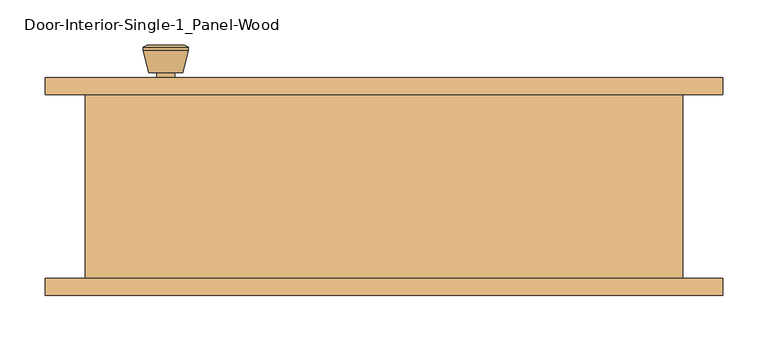
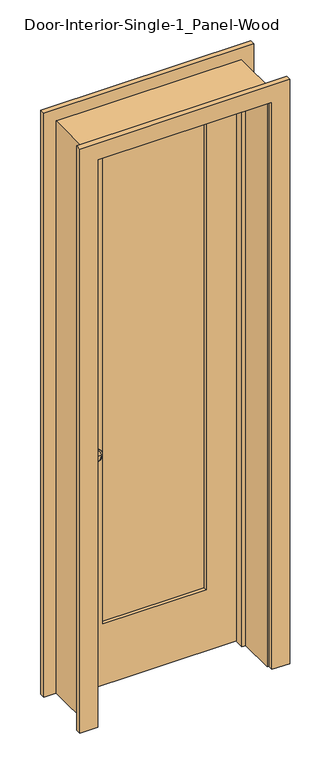
"""IFC4 building model written with IfcOpenShell, lengths in millimetres: door geometry, Door-Interior-Single-1_Panel-Wood."""

from ifc_helpers import new_model, si_unit, point, frame, frame_2d, origin, place, context, project, spatial, polyline, circle_curve, trimmed, segment, composite_curve, outline, extrude, faceted_brep, source, transform, mapped, element, save
from ifc_brep_helpers import plane_surface, cylinder_surface, revolved_surface, advanced_brep


def door_interior_single_1_panel_wood_5fe0af8f(model_context):
    return source(origin(), model_context, "Body", "SolidModel", [
        advanced_brep(
        [(-241.3, 57.5, 914.4), (-231.3, 57.5, 914.4), (-251.3, 57.5, 914.4), (-220.8241324, 8.5, 914.4), (-241.3, 8.5, 914.4), (-261.7758676, 8.5, 914.4), (-216.3, 10.3278681, 914.4), (-266.3, 10.3278681, 914.4), (-216.3, 13.7915463, 914.4), (-266.3, 13.7915463, 914.4), (-222.663764, 38.5, 914.4), (-259.936236, 38.5, 914.4), (-231.3, 38.5, 914.4), (-251.3, 38.5, 914.4)],
        [
            (0, 1),
            (1, 2, circle_curve(frame((-241.3, 57.5, 914.4), z_axis=(0.0, 1.0, 0.0), x_axis=(-1.0, 0.0, 0.0)), 10.0)),
            (2, 0),
            (2, 1, circle_curve(frame((-241.3, 57.5, 914.4), z_axis=(0.0, 1.0, 0.0), x_axis=(-1.0, 0.0, 0.0)), 10.0)),
            (3, 4),
            (4, 5),
            (5, 3, circle_curve(frame((-241.3, 8.5, 914.4), z_axis=(0.0, -1.0, 0.0), x_axis=(-1.0, 0.0, 0.0)), 20.4758676)),
            (3, 5, circle_curve(frame((-241.3, 8.5, 914.4), z_axis=(0.0, -1.0, 0.0), x_axis=(-1.0, 0.0, 0.0)), 20.4758676)),
            (6, 3),
            (5, 7),
            (7, 6, circle_curve(frame((-241.3, 10.3278681, 914.4), z_axis=(0.0, -1.0, 0.0), x_axis=(-1.0, 0.0, 0.0)), 25.0)),
            (6, 7, circle_curve(frame((-241.3, 10.3278681, 914.4), z_axis=(0.0, -1.0, 0.0), x_axis=(-1.0, 0.0, 0.0)), 25.0)),
            (8, 6),
            (7, 9),
            (9, 8, circle_curve(frame((-241.3, 13.7915463, 914.4), z_axis=(0.0, -1.0, 0.0), x_axis=(-1.0, 0.0, 0.0)), 25.0)),
            (8, 9, circle_curve(frame((-241.3, 13.7915463, 914.4), z_axis=(0.0, -1.0, 0.0), x_axis=(-1.0, 0.0, 0.0)), 25.0)),
            (10, 8),
            (9, 11),
            (11, 10, circle_curve(frame((-241.3, 38.5, 914.4), z_axis=(0.0, -1.0, 0.0), x_axis=(-1.0, 0.0, 0.0)), 18.636236)),
            (10, 11, circle_curve(frame((-241.3, 38.5, 914.4), z_axis=(0.0, -1.0, 0.0), x_axis=(-1.0, 0.0, 0.0)), 18.636236)),
            (12, 10),
            (11, 13),
            (13, 12, circle_curve(frame((-241.3, 38.5, 914.4), z_axis=(0.0, -1.0, 0.0), x_axis=(-1.0, 0.0, 0.0)), 10.0)),
            (12, 13, circle_curve(frame((-241.3, 38.5, 914.4), z_axis=(0.0, -1.0, 0.0), x_axis=(-1.0, 0.0, 0.0)), 10.0)),
            (1, 12),
            (13, 2),
        ],
        [
            plane_surface(frame((-241.3, 57.5, 914.4), z_axis=(0.0, 1.0, 0.0), x_axis=(-1.0, 0.0, 0.0))),
            plane_surface(frame((-241.3, 8.5, 914.4), z_axis=(0.0, -1.0, 0.0), x_axis=(-1.0, 0.0, 0.0))),
            revolved_surface(polyline([(-261.7758676, 8.5, 914.4), (-266.3, 10.3278681, 914.4)]), (-241.3, 57.5, 914.4), (0.0, 1.0, 0.0)),
            cylinder_surface(frame((-241.3, 57.5, 914.4), z_axis=(0.0, 1.0, 0.0), x_axis=(-1.0, 0.0, 0.0)), 25.0),
            revolved_surface(polyline([(-266.3, 13.7915463, 914.4), (-259.936236, 38.5, 914.4)]), (-241.3, 57.5, 914.4), (0.0, 1.0, 0.0)),
            plane_surface(frame((-241.3, 38.5, 914.4), z_axis=(0.0, 1.0, 0.0), x_axis=(-1.0, 0.0, 0.0))),
            cylinder_surface(frame((-241.3, 57.5, 914.4), z_axis=(0.0, 1.0, 0.0), x_axis=(-1.0, 0.0, 0.0)), 10.0),
        ],
        [
            (0, [[1, 2, 3]]),
            (0, [[-3, 4, -1]]),
            (1, [[5, 6, 7]]),
            (1, [[-6, -5, 8]]),
            (2, [[9, -7, 10, 11]]),
            (2, [[-10, -8, -9, 12]]),
            (3, [[13, -11, 14, 15]]),
            (3, [[-14, -12, -13, 16]]),
            (4, [[17, -15, 18, 19]]),
            (4, [[-18, -16, -17, 20]]),
            (5, [[21, -19, 22, 23]]),
            (5, [[-22, -20, -21, 24]]),
            (6, [[25, -23, 26, -2]]),
            (6, [[-26, -24, -25, -4]]),
        ],
    ),
        extrude(outline(composite_curve([segment(trimmed(circle_curve(frame_2d((914.4, -241.3)), 30.0), [point((914.4, -271.3))], [point((914.4, -211.3))], False, "CARTESIAN"), True, "CONTINUOUS"), segment(trimmed(circle_curve(frame_2d((914.4, -241.3)), 30.0), [point((914.4, -211.3))], [point((914.4, -271.3))], False, "CARTESIAN"), True, "CONTINUOUS")], self_intersect=False)), frame((0.0, 57.5, 0.0), z_axis=(0.0, 1.0, 0.0), x_axis=(0.0, 0.0, 1.0)), (0.0, 0.0, 1.0), 6.0),
        advanced_brep(
        [(-241.3, 104.425, 914.4), (-251.3, 104.425, 914.4), (-231.3, 104.425, 914.4), (-220.8241324, 153.425, 914.4), (-261.7758676, 153.425, 914.4), (-241.3, 153.425, 914.4), (-216.3, 151.5971319, 914.4), (-266.3, 151.5971319, 914.4), (-216.3, 148.1334537, 914.4), (-266.3, 148.1334537, 914.4), (-222.663764, 123.425, 914.4), (-259.936236, 123.425, 914.4), (-231.3, 123.425, 914.4), (-251.3, 123.425, 914.4)],
        [
            (0, 1),
            (1, 2, circle_curve(frame((-241.3, 104.425, 914.4), z_axis=(0.0, -1.0, 0.0), x_axis=(-1.0, 0.0, 0.0)), 10.0)),
            (2, 0),
            (2, 1, circle_curve(frame((-241.3, 104.425, 914.4), z_axis=(0.0, -1.0, 0.0), x_axis=(-1.0, 0.0, 0.0)), 10.0)),
            (3, 4, circle_curve(frame((-241.3, 153.425, 914.4), z_axis=(0.0, 1.0, 0.0), x_axis=(-1.0, 0.0, 0.0)), 20.4758676)),
            (4, 5),
            (5, 3),
            (4, 3, circle_curve(frame((-241.3, 153.425, 914.4), z_axis=(0.0, 1.0, 0.0), x_axis=(-1.0, 0.0, 0.0)), 20.4758676)),
            (6, 7, circle_curve(frame((-241.3, 151.5971319, 914.4), z_axis=(0.0, 1.0, 0.0), x_axis=(-1.0, 0.0, 0.0)), 25.0)),
            (7, 4),
            (3, 6),
            (7, 6, circle_curve(frame((-241.3, 151.5971319, 914.4), z_axis=(0.0, 1.0, 0.0), x_axis=(-1.0, 0.0, 0.0)), 25.0)),
            (8, 9, circle_curve(frame((-241.3, 148.1334537, 914.4), z_axis=(0.0, 1.0, 0.0), x_axis=(-1.0, 0.0, 0.0)), 25.0)),
            (9, 7),
            (6, 8),
            (9, 8, circle_curve(frame((-241.3, 148.1334537, 914.4), z_axis=(0.0, 1.0, 0.0), x_axis=(-1.0, 0.0, 0.0)), 25.0)),
            (10, 11, circle_curve(frame((-241.3, 123.425, 914.4), z_axis=(0.0, 1.0, 0.0), x_axis=(-1.0, 0.0, 0.0)), 18.636236)),
            (11, 9),
            (8, 10),
            (11, 10, circle_curve(frame((-241.3, 123.425, 914.4), z_axis=(0.0, 1.0, 0.0), x_axis=(-1.0, 0.0, 0.0)), 18.636236)),
            (12, 13, circle_curve(frame((-241.3, 123.425, 914.4), z_axis=(0.0, 1.0, 0.0), x_axis=(-1.0, 0.0, 0.0)), 10.0)),
            (13, 11),
            (10, 12),
            (13, 12, circle_curve(frame((-241.3, 123.425, 914.4), z_axis=(0.0, 1.0, 0.0), x_axis=(-1.0, 0.0, 0.0)), 10.0)),
            (1, 13),
            (12, 2),
        ],
        [
            plane_surface(frame((-241.3, 104.425, 914.4), z_axis=(0.0, -1.0, 0.0), x_axis=(-1.0, 0.0, 0.0))),
            plane_surface(frame((-241.3, 153.425, 914.4), z_axis=(0.0, 1.0, 0.0), x_axis=(-1.0, 0.0, 0.0))),
            revolved_surface(polyline([(-261.7758676, 153.425, 914.4), (-266.3, 151.5971319, 914.4)]), (-241.3, 104.425, 914.4), (0.0, -1.0, 0.0)),
            cylinder_surface(frame((-241.3, 104.425, 914.4), z_axis=(0.0, -1.0, 0.0), x_axis=(-1.0, 0.0, 0.0)), 25.0),
            revolved_surface(polyline([(-266.3, 148.1334537, 914.4), (-259.936236, 123.425, 914.4)]), (-241.3, 104.425, 914.4), (0.0, -1.0, 0.0)),
            plane_surface(frame((-241.3, 123.425, 914.4), z_axis=(0.0, -1.0, 0.0), x_axis=(-1.0, 0.0, 0.0))),
            cylinder_surface(frame((-241.3, 104.425, 914.4), z_axis=(0.0, -1.0, 0.0), x_axis=(-1.0, 0.0, 0.0)), 10.0),
        ],
        [
            (0, [[1, 2, 3]]),
            (0, [[-3, 4, -1]]),
            (1, [[5, 6, 7]]),
            (1, [[8, -7, -6]]),
            (2, [[9, 10, -5, 11]]),
            (2, [[12, -11, -8, -10]]),
            (3, [[13, 14, -9, 15]]),
            (3, [[16, -15, -12, -14]]),
            (4, [[17, 18, -13, 19]]),
            (4, [[20, -19, -16, -18]]),
            (5, [[21, 22, -17, 23]]),
            (5, [[24, -23, -20, -22]]),
            (6, [[-2, 25, -21, 26]]),
            (6, [[-4, -26, -24, -25]]),
        ],
    ),
        extrude(outline(composite_curve([segment(trimmed(circle_curve(frame_2d((914.4, -241.3)), 30.0), [point((914.4, -271.3))], [point((914.4, -211.3))], False, "CARTESIAN"), True, "CONTINUOUS"), segment(trimmed(circle_curve(frame_2d((914.4, -241.3)), 30.0), [point((914.4, -211.3))], [point((914.4, -271.3))], False, "CARTESIAN"), True, "CONTINUOUS")], self_intersect=False)), frame((0.0, 98.425, 0.0), z_axis=(0.0, 1.0, 0.0), x_axis=(0.0, 0.0, 1.0)), (0.0, 0.0, 1.0), 6.0),
        faceted_brep([(330.2, 98.425, 0.0), (330.2, -104.775, 0.0), (304.8, -104.775, 0.0), (304.8, 28.575, 0.0), (292.1, 28.575, 0.0), (292.1, 63.5, 0.0), (304.8, 63.5, 0.0), (304.8, 98.425, 0.0), (330.2, 98.425, 2159.0), (330.2, -104.775, 2159.0), (-330.2, -104.775, 2159.0), (-330.2, -104.775, 0.0), (-304.8, -104.775, 0.0), (-304.8, -104.775, 2133.6), (304.8, -104.775, 2133.6), (304.8, 28.575, 2133.6), (-304.8, 28.575, 2133.6), (-304.8, 28.575, 0.0), (-292.1, 28.575, 0.0), (-292.1, 28.575, 2120.9), (292.1, 28.575, 2120.9), (292.1, 63.5, 2120.9), (-292.1, 63.5, 2120.9), (-292.1, 63.5, 0.0), (-304.8, 63.5, 0.0), (-304.8, 63.5, 2133.6), (304.8, 63.5, 2133.6), (304.8, 98.425, 2133.6), (-304.8, 98.425, 2133.6), (-304.8, 98.425, 0.0), (-330.2, 98.425, 0.0), (-330.2, 98.425, 2159.0)], [[[0, 1, 2, 3, 4, 5, 6, 7]], [[1, 0, 8, 9]], [[2, 1, 9, 10, 11, 12, 13, 14]], [[3, 2, 14, 15]], [[4, 3, 15, 16, 17, 18, 19, 20]], [[5, 4, 20, 21]], [[6, 5, 21, 22, 23, 24, 25, 26]], [[7, 6, 26, 27]], [[0, 7, 27, 28, 29, 30, 31, 8]], [[9, 8, 31, 10]], [[15, 14, 13, 16]], [[21, 20, 19, 22]], [[27, 26, 25, 28]], [[30, 29, 24, 23, 18, 17, 12, 11]], [[10, 31, 30, 11]], [[16, 13, 12, 17]], [[22, 19, 18, 23]], [[28, 25, 24, 29]]]),
        extrude(outline(polyline([(2133.6, -304.8), (0.0, -304.8), (0.0, 304.8), (2133.6, 304.8), (2133.6, -304.8)]), holes=[polyline([(2014.5375, -184.15), (2014.5375, 184.15), (231.775, 184.15), (231.775, -184.15), (2014.5375, -184.15)])]), frame((0.0, 63.5, 0.0), z_axis=(0.0, 1.0, 0.0), x_axis=(0.0, 0.0, 1.0)), (0.0, 0.0, 1.0), 34.925),
        extrude(outline(polyline([(184.15, 75.1416667), (-184.15, 75.1416667), (-184.15, 86.7833333), (184.15, 86.7833333), (184.15, 75.1416667)])), frame((0.0, 0.0, 231.775), z_axis=(0.0, 0.0, 1.0), x_axis=(1.0, 0.0, 0.0)), (0.0, 0.0, 1.0), 1782.7625),
        extrude(outline(polyline([(0.0, 311.15), (0.0, 374.65), (2203.45, 374.65), (2203.45, -374.65), (0.0, -374.65), (0.0, -311.15), (2139.95, -311.15), (2139.95, 311.15), (0.0, 311.15)])), frame((0.0, 98.425, 0.0), z_axis=(0.0, 1.0, 0.0), x_axis=(0.0, 0.0, 1.0)), (0.0, 0.0, 1.0), 19.05),
        extrude(outline(polyline([(0.0, 311.15), (0.0, 374.65), (2203.45, 374.65), (2203.45, -374.65), (0.0, -374.65), (0.0, -311.15), (2139.95, -311.15), (2139.95, 311.15), (0.0, 311.15)])), frame((0.0, -123.825, 0.0), z_axis=(0.0, 1.0, 0.0), x_axis=(0.0, 0.0, 1.0)), (0.0, 0.0, 1.0), 19.05),
    ])


if __name__ == "__main__":
    model = new_model("IFC4")
    model_context = context("Model", 3, world=origin())
    ifc_project = project(units=[si_unit("LENGTHUNIT", "METRE", prefix="MILLI")], contexts=[model_context])
    site = spatial("IfcSite", under=ifc_project)
    building = spatial("IfcBuilding", under=site)
    placement = place(None, origin())
    door_interior_single_1_panel_wood_shape = door_interior_single_1_panel_wood_5fe0af8f(model_context)
    element("IfcDoor", 1, ObjectType="Door-Interior-Single-1_Panel-Wood", at=placement, inside=building, context=model_context, shape_type="MappedRepresentation", body=[
        mapped(door_interior_single_1_panel_wood_shape, transform((0.0, 0.0, 0.0), x_axis=(1.0, 0.0, 0.0), y_axis=(0.0, 1.0, 0.0), z_axis=(0.0, 0.0, 1.0))),
    ])
    save(model, "model.ifc")

# Revit data of these elements
# Type "Door-Interior-Single-1_Panel-Wood"
#   Type Mark = "12"
#   Assembly Code = "C1020300"
#   Analytic Construction = "Wooden"
#   Top Rail = 0' - 4 11/16"
#   Thickness = 0' - 1 3/8"
#   Thermal Resistance (R) = 2.5876 (h·ft²·°F)/BTU
#   Swing Angle [instance default] = 90.00°
#   Stiles = 0' - 4 3/4"
#   Rough Width = 2' - 2"
#   Rough Height = 7' - 1"
#   Height = 7' - 0"
#   Width = 2' - 0"
#   Heat Transfer Coefficient (U) = 0.3865 BTU/(h·ft²·°F)
#   Bottom Rail = 0' - 9 1/8"
#   Trim Material = Cherry
#   Panel Material = Cherry
#   Frame Material = Cherry
#   Door Handle Material = Aluminum
#   Visual Light Transmittance = 0
#   Solar Heat Gain Coefficient = 0
#   Wall Closure = (empty or 0)
#   Function = (empty or 0)
# Element 1 (IfcDoor, "Door-Interior-Single-1_Panel-Wood")
#   Materials on its faces: "Cherry", "Aluminum"
# Materials
#   "Cherry": class "Wood", colour RGB 226 177 128, transparency 0, Description = "Prunus Serotina", Cost = 0
#   "Aluminum": class "Metal", colour RGB 247 247 247, transparency 0, Description = "Aluminum 6061", Cost = 0
